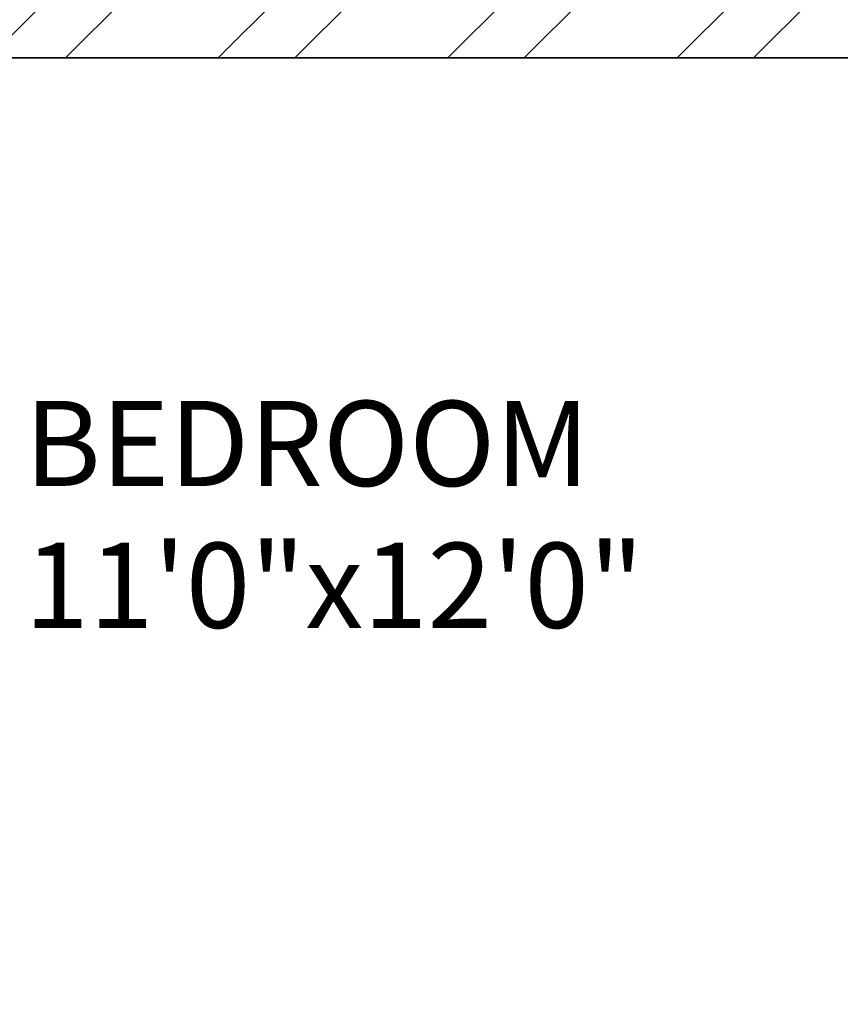
# Model space of a CAD drawing. Units: inches. Extents: x 1962 to 2771, y 1245 to 2660.
# Tile 50 of 114: x 2112 to 2160, y 2122 to 2180. Entities that reach past the tile are written whole.
import ezdxf

# ---------------------------------------------------------------- set-up
doc = ezdxf.new("R2010")
doc.units = ezdxf.units.IN
for name, color, linetype, lineweight in [('A-ANNO-DIMS', 2, 'Continuous', 18), ('A-AREA-IDEN', 7, 'Continuous', 18), ('A-WALL', 7, 'Continuous', 35), ('A-WALL-PATT', 252, 'Continuous', 13)]:
    doc.layers.add(name, color=color, linetype=linetype, lineweight=lineweight)
doc.styles.get("Standard").update_dxf_attribs({"font": 'arial.ttf'})
doc.dimstyles.get("Standard").update_dxf_attribs({"dimtxt": 0.18, "dimasz": 0.18, "dimexe": 0.18, "dimexo": 0.0625, "dimgap": 0.09, "dimtad": 0, "dimtih": 1, "dimtoh": 1, "dimdec": 4, "dimzin": 0, "dimdsep": 46, "dimtxsty": 'Standard', "dimcen": 0.09, "dimadec": 0, "dimazin": 0, "dimtfac": 1, "dimtdec": 4, "dimtofl": 0, "dimtmove": 0, "dimatfit": 3, "dimfxl": 1, "dimtolj": 1, "dimtzin": 0, "dimarcsym": 0})

# ---------------------------------------------------------------- blocks, each defined once
blk = doc.blocks.new('*D40')
at = {"layer": 'A-ANNO-DIMS', "color": 0, "lineweight": -2, "transparency": 16777216}
for p, q in [((2072.02, 2033.906), (2072.02, 2583.474)), ((2072.2, 2583.294), (2366.02, 2583.294)), ((2660.627, 2583.294), (2366.808, 2583.294)), ((2660.807, 2524.406), (2660.807, 2583.474))]:
    blk.add_line(p, q, dxfattribs=at)
at = {"layer": 'A-ANNO-DIMS', "color": 0, "transparency": 16777216}
for points in [[(2072.2, 2583.324), (2072.2, 2583.264), (2072.02, 2583.294)], [(2660.627, 2583.324), (2660.627, 2583.264), (2660.807, 2583.294)]]:
    blk.add_solid(points, dxfattribs=at)
at = {"layer": 'Defpoints', "color": 0, "transparency": 16777216}
for p in [(2660.807, 2583.294), (2660.807, 2524.344), (2072.02, 2033.844)]:
    blk.add_point(p, dxfattribs=at)
at = {"layer": 'A-ANNO-DIMS', "color": 0, "transparency": 16777216, "insert": (2366.414, 2583.294), "char_height": 0.18, "attachment_point": 5}
blk.add_mtext('\\A1;588.8', dxfattribs=at)

msp = doc.modelspace()

# ---------------------------------------------------------------- hatches: boundary and pattern name
at = {"layer": 'A-WALL-PATT'}
h = msp.add_hatch(dxfattribs=at)
h.set_pattern_fill('ANSI32', color=256)
h.paths.add_polyline_path([(2090.8074, 2467.3437), (2141.6481, 2467.3437), (2141.6481, 2469.5937), (2141.6481, 2471.8437), (2086.3074, 2471.8437), (2086.3074, 2422.5333), (2090.8074, 2422.5333)])
h.paths.add_polyline_path([(2282.7664, 2471.8437), (2204.8982, 2471.8437), (2204.8982, 2467.3437), (2234.8074, 2467.3437), (2234.8074, 2311.3437), (2228.7492, 2311.3437), (2228.7492, 2306.8437), (2234.8074, 2306.8437), (2331.9227, 2306.8437), (2331.9227, 2309.0937), (2331.9227, 2311.3437), (2239.3074, 2311.3437), (2239.3074, 2467.3437), (2282.7664, 2467.3437), (2282.7664, 2469.5937)])
h.paths.add_polyline_path([(2471.4531, 2519.8437), (2552.011, 2519.8437), (2564.3996, 2519.8437), (2564.3996, 2511.1389), (2568.8996, 2511.1389), (2568.8996, 2524.3437), (2466.9531, 2524.3437), (2466.9531, 2471.8437), (2450.0749, 2471.8437), (2446.4672, 2471.8437), (2446.4672, 2467.3437), (2450.0749, 2467.3437), (2475.9988, 2467.3437), (2475.9988, 2469.5937), (2475.9988, 2471.8437), (2471.4531, 2471.8437)])
h.paths.add_polyline_path([(2575.2231, 2469.5937), (2575.2231, 2471.8437), (2568.8996, 2471.8437), (2568.8996, 2487.1389), (2564.3996, 2487.1389), (2564.3996, 2471.8437), (2556.511, 2471.8437), (2499.2904, 2471.8437), (2499.2904, 2467.3437), (2507.8074, 2467.3437), (2507.8074, 2311.3437), (2414.863, 2311.3437), (2414.863, 2306.8437), (2512.3074, 2306.8437), (2517.0114, 2306.8437), (2517.0114, 2309.0937), (2517.0114, 2311.3437), (2512.3074, 2311.3437), (2512.3074, 2467.3437), (2575.2231, 2467.3437)])
h.paths.add_polyline_path([(2660.8074, 2471.8437), (2600.9602, 2471.8437), (2600.9602, 2467.3437), (2656.3074, 2467.3437), (2656.3074, 2432.5704), (2660.8074, 2432.5704)])
h.paths.add_polyline_path([(2660.8074, 2372.5704), (2656.3074, 2372.5704), (2656.3074, 2311.3437), (2600.276, 2311.3437), (2600.276, 2309.0937), (2600.276, 2306.8437), (2656.3074, 2306.8437), (2656.3074, 2296.2593), (2660.8074, 2296.2593)])
h.paths.add_polyline_path([(2572.3074, 2306.8437), (2577.1385, 2306.8437), (2577.1385, 2311.3437), (2551.082, 2311.3437), (2551.082, 2306.8437), (2567.8074, 2306.8437), (2567.8074, 2258.8437), (2540.0574, 2258.8437), (2540.0574, 2256.5937), (2540.0574, 2254.3437), (2567.8074, 2254.3437), (2656.3074, 2254.3437), (2656.3074, 2236.9085), (2660.8074, 2236.9085), (2660.8074, 2272.2593), (2656.3074, 2272.2593), (2656.3074, 2258.8437), (2572.3074, 2258.8437)])
h.paths.add_polyline_path([(2512.3074, 2254.3437), (2518.8716, 2254.3437), (2518.8716, 2256.5937), (2518.8716, 2258.8437), (2507.8074, 2258.8437), (2507.8074, 2177.8437), (2567.8074, 2177.8437), (2567.8074, 2172.9628), (2572.3074, 2172.9628), (2572.3074, 2177.8437), (2656.3074, 2177.8437), (2656.3074, 2166.4846), (2660.8074, 2166.4846), (2660.8074, 2200.9085), (2656.3074, 2200.9085), (2656.3074, 2182.3437), (2512.3074, 2182.3437)])
h.paths.add_polyline_path([(2656.3074, 2129.8437), (2572.3074, 2129.8437), (2572.3074, 2150.3044), (2570.0574, 2150.3044), (2567.8074, 2150.3044), (2567.8074, 2129.8437), (2507.8074, 2129.8437), (2507.8074, 2116.3027), (2510.0574, 2116.3027), (2512.3074, 2116.3027), (2512.3074, 2125.3437), (2567.8074, 2125.3437), (2572.3074, 2125.3437), (2656.3074, 2125.3437)])
h.paths.add_polyline_path([(2090.8074, 2362.5333), (2086.3074, 2362.5333), (2086.3074, 2298.6242), (2090.8074, 2298.6242), (2090.8074, 2306.8437), (2174.8074, 2306.8437), (2174.8074, 2286.4178), (2179.3074, 2286.4178), (2179.3074, 2306.8437), (2192.8641, 2306.8437), (2192.8641, 2309.0937), (2192.8641, 2311.3437), (2090.8074, 2311.3437)])
h.paths.add_polyline_path([(2209.156, 2258.8437), (2179.3074, 2258.8437), (2179.3074, 2263.2236), (2177.0574, 2263.2236), (2174.8074, 2263.2236), (2174.8074, 2258.8437), (2090.8074, 2258.8437), (2090.8074, 2274.6242), (2086.3074, 2274.6242), (2086.3074, 2238.2967), (2088.5574, 2238.2967), (2090.8074, 2238.2967), (2090.8074, 2254.3437), (2209.156, 2254.3437)])
h.paths.add_polyline_path([(2090.8074, 2177.8437), (2234.8074, 2177.8437), (2234.8074, 2173.1428), (2239.3074, 2173.1428), (2239.3074, 2258.8437), (2230.8442, 2258.8437), (2230.8442, 2256.5937), (2230.8442, 2254.3437), (2234.8074, 2254.3437), (2234.8074, 2182.3437), (2090.8074, 2182.3437), (2090.8074, 2202.2967), (2086.3074, 2202.2967), (2086.3074, 2140.0389), (2090.8074, 2140.0389)])
h.paths.add_polyline_path([(2090.8074, 2080.0389), (2086.3074, 2080.0389), (2086.3074, 2033.8437), (2090.8074, 2033.8437)], flags=17)
h.paths.add_polyline_path([(2244.9405, 2033.8437), (2239.3074, 2033.8437), (2239.3074, 2142.0665), (2237.2592, 2142.0665), (2234.8074, 2142.0665), (2234.8074, 2033.8437), (2090.8074, 2033.8437), (2076.5204, 2033.8437), (2072.0204, 2033.8437), (2072.0204, 2000.4493), (2076.5204, 2000.4493), (2076.5204, 2029.3437), (2090.8074, 2029.3437), (2244.9405, 2029.3437), (2244.9405, 2031.5937)])
h.paths.add_polyline_path([(2234.8074, 1933.3437), (2076.5204, 1933.3437), (2076.5204, 1952.4493), (2074.2704, 1952.4493), (2072.0204, 1952.4493), (2072.0204, 1933.3437), (2072.0204, 1928.8437), (2234.8074, 1928.8437)])
h.paths.add_polyline_path([(2090.8074, 1928.8437), (2086.3074, 1928.8437), (2086.3074, 1906.5013), (2090.8074, 1906.5013)])
h.paths.add_polyline_path([(2090.8074, 1846.5013), (2086.3074, 1846.5013), (2086.3074, 1769.9917), (2088.5574, 1769.9917), (2090.8074, 1769.9917), (2090.8074, 1780.3437), (2234.8074, 1780.3437), (2234.8074, 1708.3437), (2230.3764, 1708.3437), (2230.3764, 1703.8437), (2239.3074, 1703.8437), (2239.3074, 1792.6669), (2237.0574, 1792.6669), (2234.8074, 1792.6669), (2234.8074, 1784.8437), (2090.8074, 1784.8437)])
h.paths.add_polyline_path([(2239.3074, 1928.8437), (2244.9405, 1928.8437), (2244.9405, 1931.0937), (2244.9405, 1933.3437), (2234.8074, 1933.3437), (2234.8074, 1928.8437), (2234.8074, 1825.5949), (2239.3074, 1825.5949)])
h.paths.add_polyline_path([(2148.0425, 1649.0937), (2148.0425, 1651.3437), (2090.8074, 1651.3437), (2090.8074, 1646.8437), (2148.0425, 1646.8437)], flags=0)
h.paths.add_polyline_path([(2207.5601, 1708.3437), (2090.8074, 1708.3437), (2090.8074, 1703.8437), (2174.8074, 1703.8437), (2174.8074, 1651.3437), (2170.4457, 1651.3437), (2170.4457, 1646.8437), (2195.9924, 1646.8437), (2195.9924, 1649.0937), (2195.9924, 1651.3437), (2179.3074, 1651.3437), (2179.3074, 1703.8437), (2207.5601, 1703.8437), (2207.5601, 1706.0937)])
h.paths.add_polyline_path([(2090.8074, 1733.9917), (2086.3074, 1733.9917), (2086.3074, 1696.1032), (2088.5574, 1696.1032), (2090.8074, 1696.1032)])
h.paths.add_polyline_path([(2090.8074, 1672.1032), (2086.3074, 1672.1032), (2086.3074, 1600.3335), (2090.8074, 1600.3335)])
h.paths.add_polyline_path([(2090.8074, 1540.3335), (2086.3074, 1540.3335), (2086.3074, 1486.3437), (2139.6766, 1486.3437), (2139.6766, 1490.8437), (2090.8074, 1490.8437)])
h.paths.add_polyline_path([(2302.3876, 1490.8437), (2239.3074, 1490.8437), (2239.3074, 1646.8437), (2335.9994, 1646.8437), (2335.9994, 1651.3437), (2229.884, 1651.3437), (2229.884, 1646.8437), (2234.8074, 1646.8437), (2234.8074, 1490.8437), (2202.7103, 1490.8437), (2202.7103, 1488.5937), (2202.7103, 1486.3437), (2275.0699, 1486.3437), (2275.0699, 1475.772), (2279.5699, 1475.772), (2279.5699, 1486.3437), (2302.3876, 1486.3437)])
h.paths.add_polyline_path([(2279.5699, 1451.772), (2275.0699, 1451.772), (2275.0699, 1438.3437), (2174.8074, 1438.3437), (2174.8074, 1486.3437), (2179.7922, 1486.3437), (2179.7922, 1490.8437), (2163.3585, 1490.8437), (2163.3585, 1488.5937), (2163.3585, 1486.3437), (2170.3074, 1486.3437), (2170.3074, 1433.8437), (2279.5699, 1433.8437)])
h.paths.add_polyline_path([(2427.2363, 1490.8437), (2375.8074, 1490.8437), (2375.8074, 1646.8437), (2381.6401, 1646.8437), (2381.6401, 1651.3437), (2365.887, 1651.3437), (2365.887, 1649.0937), (2365.887, 1646.8437), (2371.3074, 1646.8437), (2371.3074, 1490.8437), (2327.5627, 1490.8437), (2327.5627, 1488.5937), (2327.5627, 1486.3437), (2371.3074, 1486.3437), (2371.3074, 1433.8437), (2375.8074, 1433.8437), (2375.8074, 1486.3437), (2427.2363, 1486.3437)])
h.paths.add_polyline_path([(2512.3074, 1646.8437), (2519.4351, 1646.8437), (2519.4351, 1649.0937), (2519.4351, 1651.3437), (2507.8074, 1651.3437), (2416.0063, 1651.3437), (2416.0063, 1649.0937), (2416.0063, 1646.8437), (2507.8074, 1646.8437), (2507.8074, 1490.8437), (2497.0532, 1490.8437), (2497.0532, 1488.5937), (2497.0532, 1486.3437), (2574.9344, 1486.3437), (2574.9344, 1476.0181), (2579.4344, 1476.0181), (2579.4344, 1486.3437), (2584.4872, 1486.3437), (2584.3074, 1490.8437), (2512.3074, 1490.8437)])
h.paths.add_polyline_path([(2470.5091, 1486.3437), (2473.9767, 1486.3437), (2473.9767, 1490.8437), (2449.6605, 1490.8437), (2449.6605, 1488.5937), (2449.6605, 1486.3437), (2466.0091, 1486.3437), (2466.0091, 1433.8437), (2470.5091, 1433.8437), (2579.4344, 1433.8437), (2579.4344, 1452.0181), (2574.9344, 1452.0181), (2574.9344, 1438.3437), (2554.5091, 1438.3437), (2470.5091, 1438.3437)])
h.paths.add_polyline_path([(2656.3074, 1490.8437), (2611.86, 1490.8437), (2611.86, 1486.3437), (2656.3074, 1486.3437)])
h.paths.add_polyline_path([(2660.8074, 1532.7007), (2658.5574, 1532.7007), (2656.3074, 1532.7007), (2656.3074, 1486.3437), (2660.8074, 1486.3437)])
h.paths.add_polyline_path([(2660.8074, 1664.9663), (2656.3074, 1664.9663), (2656.3074, 1651.3437), (2602.2313, 1651.3437), (2602.2313, 1646.8437), (2656.3074, 1646.8437), (2656.3074, 1592.7007), (2660.8074, 1592.7007)])
h.paths.add_polyline_path([(2660.8074, 1724.5221), (2656.3074, 1724.5221), (2656.3074, 1703.8437), (2542.4725, 1703.8437), (2542.4725, 1699.3437), (2567.8074, 1699.3437), (2567.8074, 1651.3437), (2552.7766, 1651.3437), (2552.7766, 1649.0937), (2552.7766, 1646.8437), (2577.2878, 1646.8437), (2577.2878, 1649.0937), (2577.2878, 1651.3437), (2572.3074, 1651.3437), (2572.3074, 1699.3437), (2656.3074, 1699.3437), (2656.3074, 1688.9663), (2660.8074, 1688.9663)])
h.paths.add_polyline_path([(2660.8074, 1880.6524), (2656.3074, 1880.6524), (2656.3074, 1832.8437), (2512.3074, 1832.8437), (2512.3074, 1837.8959), (2507.8074, 1837.8959), (2507.8074, 1828.3437), (2567.8074, 1828.3437), (2567.8074, 1804.3437), (2572.3074, 1804.3437), (2572.3074, 1828.3437), (2656.3074, 1828.3437), (2656.3074, 1818.6778), (2660.8074, 1818.6778)])
h.paths.add_polyline_path([(2660.8074, 1794.6778), (2656.3074, 1794.6778), (2656.3074, 1780.3437), (2572.3074, 1780.3437), (2572.3074, 1783.0303), (2570.0574, 1783.0303), (2567.8074, 1783.0303), (2567.8074, 1780.3437), (2507.8074, 1780.3437), (2507.8074, 1699.3437), (2517.8858, 1699.3437), (2517.8858, 1701.5937), (2517.8858, 1703.8437), (2512.3074, 1703.8437), (2512.3074, 1775.8437), (2656.3074, 1775.8437), (2656.3074, 1760.5221), (2660.8074, 1760.5221)])
h.paths.add_polyline_path([(2660.8074, 1981.3437), (2660.8074, 2020.2808), (2658.5574, 2020.2808), (2656.3074, 2020.2808), (2656.3074, 1981.3437), (2512.3074, 1981.3437), (2512.3074, 2086.6996), (2507.8074, 2086.6996), (2507.8074, 1981.3437), (2375.8074, 1981.3437), (2375.8074, 1986.8505), (2373.5574, 1986.8505), (2371.3074, 1986.8505), (2371.3074, 1973.2607), (2375.8074, 1973.2607), (2375.8074, 1976.8437), (2507.8074, 1976.8437), (2507.8074, 1865.4281), (2510.0574, 1865.4281), (2512.3074, 1865.4281), (2512.3074, 1976.8437), (2660.8074, 1976.8437)])
h.paths.add_polyline_path([(2375.8074, 1940.297), (2373.5574, 1940.297), (2371.3074, 1940.297), (2371.3074, 1933.3437), (2278.4434, 1933.3437), (2278.4434, 1928.8437), (2371.3074, 1928.8437), (2371.3074, 1651.3437), (2375.8074, 1651.3437)])
h.paths.add_polyline_path([(2660.8074, 1976.8437), (2656.3074, 1976.8437), (2656.3074, 1940.6524), (2660.8074, 1940.6524)], flags=17)
h.paths.add_polyline_path([(2660.8074, 2142.4846), (2656.3074, 2142.4846), (2656.3074, 2080.2808), (2660.8074, 2080.2808)])
h.paths.add_polyline_path([(2381.4189, 2311.3437), (2375.8074, 2311.3437), (2375.8074, 2467.3437), (2424.7242, 2467.3437), (2424.7242, 2469.5937), (2424.7242, 2471.8437), (2375.8074, 2471.8437), (2375.8074, 2524.3437), (2371.3074, 2524.3437), (2371.3074, 2471.8437), (2307.2097, 2471.8437), (2307.2097, 2467.3437), (2371.3074, 2467.3437), (2371.3074, 2311.3437), (2366.8901, 2311.3437), (2366.8901, 2306.8437), (2371.3074, 2306.8437), (2371.3074, 2033.8437), (2279.6589, 2033.8437), (2279.6589, 2029.3437), (2371.3074, 2029.3437), (2371.3074, 2014.2598), (2375.8074, 2014.2598), (2375.8074, 2306.8437), (2381.4189, 2306.8437)])
h.paths.add_polyline_path([(2263.3074, 2524.3437), (2170.3074, 2524.3437), (2170.3074, 2519.8437), (2170.3074, 2471.8437), (2165.0312, 2471.8437), (2165.0312, 2467.3437), (2179.6721, 2467.3437), (2179.6721, 2469.5161), (2179.6721, 2471.8437), (2174.8074, 2471.8437), (2174.8074, 2519.8437), (2258.8074, 2519.8437), (2258.8074, 2511.6436), (2263.3074, 2511.6436)])
h.paths.add_polyline_path([(2245.0232, 1361.4123), (2492.9468, 1361.4123), (2492.9468, 1398.505), (2245.0232, 1398.505)], flags=9)
h.paths.add_polyline_path([(2388.1434, 2086.6936), (2425.0704, 2086.6936), (2425.0704, 2105.3509), (2388.1434, 2105.3509)], flags=9)
h.paths.add_polyline_path([(2404.922, 2242.6744), (2445.7337, 2242.6744), (2445.7337, 2261.3318), (2404.922, 2261.3318)], flags=9)
h.paths.add_polyline_path([(2269.4107, 2156.7935), (2306.3378, 2156.7935), (2306.3378, 2175.4508), (2269.4107, 2175.4508)], flags=9)
h.paths.add_polyline_path([(2269.3277, 2233.4343), (2306.2547, 2233.4343), (2306.2547, 2252.0917), (2269.3277, 2252.0917)], flags=9)
h.paths.add_polyline_path([(2431.6052, 2320.6922), (2470.4456, 2320.6922), (2470.4456, 2339.3495), (2431.6052, 2339.3495)], flags=25)
h.paths.add_polyline_path([(2249.6902, 2315.7608), (2288.5306, 2315.7608), (2288.5306, 2334.4182), (2249.6902, 2334.4182)], flags=25)
h.paths.add_polyline_path([(2096.9301, 2314.3181), (2135.7704, 2314.3181), (2135.7704, 2332.9755), (2096.9301, 2332.9755)], flags=25)
h.paths.add_polyline_path([(2134.3475, 2285.7089), (2161.4655, 2285.7089), (2161.4655, 2304.3662), (2134.3475, 2304.3662)], flags=9)
h.paths.add_polyline_path([(2126.5155, 2209.4076), (2159.9227, 2209.4076), (2159.9227, 2228.065), (2126.5155, 2228.065)], flags=25)
h.paths.add_polyline_path([(2110.5753, 2141.5299), (2149.4157, 2141.5299), (2149.4157, 2160.1872), (2110.5753, 2160.1872)], flags=25)
h.paths.add_polyline_path([(2249.8618, 1968.3317), (2286.3966, 1968.3317), (2286.3966, 1986.989), (2249.8618, 1986.989)], flags=9)
h.paths.add_polyline_path([(2395.9507, 1777.0051), (2436.7624, 1777.0051), (2436.7624, 1795.6625), (2395.9507, 1795.6625)], flags=9)
h.paths.add_polyline_path([(2398.5259, 1888.5651), (2435.0062, 1888.5651), (2435.0062, 1907.2224), (2398.5259, 1907.2224)], flags=25)
h.paths.add_polyline_path([(2259.3506, 1728.3559), (2296.2776, 1728.3559), (2296.2776, 1747.0132), (2259.3506, 1747.0132)], flags=9)
h.paths.add_polyline_path([(2271.3698, 1845.268), (2308.2968, 1845.268), (2308.2968, 1863.9253), (2271.3698, 1863.9253)], flags=9)
h.paths.add_polyline_path([(2120.9355, 1786.3027), (2159.7759, 1786.3027), (2159.7759, 1804.9601), (2120.9355, 1804.9601)], flags=25)
h.paths.add_polyline_path([(2121.3164, 1732.1043), (2154.7236, 1732.1043), (2154.7236, 1750.7616), (2121.3164, 1750.7616)], flags=25)
h.paths.add_polyline_path([(2118.3706, 1678.8997), (2147.5282, 1678.8997), (2147.5282, 1697.557), (2118.3706, 1697.557)], flags=25)
h.paths.add_polyline_path([(2385.9227, 1493.557), (2424.763, 1493.557), (2424.763, 1512.2143), (2385.9227, 1512.2143)], flags=25)
h.paths.add_polyline_path([(2248.7058, 1500.0256), (2287.5462, 1500.0256), (2287.5462, 1518.6829), (2248.7058, 1518.6829)], flags=25)
h.paths.add_polyline_path([(2104.1669, 1617.3771), (2143.0073, 1617.3771), (2143.0073, 1636.0344), (2104.1669, 1636.0344)], flags=9)
h.paths.add_polyline_path([(2096.0714, 1447.8824), (2137.3845, 1447.8824), (2137.3845, 1458.1859), (2096.0714, 1458.1859)], flags=9)
h.paths.add_polyline_path([(2180.6114, 1440.325), (2209.7689, 1440.325), (2209.7689, 1458.9823), (2180.6114, 1458.9823)], flags=25)
h.paths.add_polyline_path([(2316.1698, 1447.9637), (2357.4829, 1447.9637), (2357.4829, 1458.2673), (2316.1698, 1458.2673)], flags=9)
h.paths.add_polyline_path([(2397.6187, 1447.9637), (2438.9318, 1447.9637), (2438.9318, 1458.2673), (2397.6187, 1458.2673)], flags=9)
h.paths.add_polyline_path([(2473.0778, 1439.5953), (2502.2354, 1439.5953), (2502.2354, 1458.2527), (2473.0778, 1458.2527)], flags=25)
h.paths.add_polyline_path([(2589.7027, 1447.8819), (2631.0158, 1447.8819), (2631.0158, 1458.1855), (2589.7027, 1458.1855)], flags=9)
h.paths.add_polyline_path([(2522.4009, 1497.5285), (2561.2413, 1497.5285), (2561.2413, 1516.1859), (2522.4009, 1516.1859)], flags=25)
h.paths.add_polyline_path([(2579.6565, 1671.3482), (2608.8141, 1671.3482), (2608.8141, 1690.0056), (2579.6565, 1690.0056)], flags=25)
h.paths.add_polyline_path([(2544.7038, 1725.5064), (2578.1111, 1725.5064), (2578.1111, 1744.1637), (2544.7038, 1744.1637)], flags=25)
h.paths.add_polyline_path([(2578.1191, 1807.472), (2607.2766, 1807.472), (2607.2766, 1826.1293), (2578.1191, 1826.1293)], flags=25)
h.paths.add_polyline_path([(2595.0614, 1835.1839), (2633.9018, 1835.1839), (2633.9018, 1853.8413), (2595.0614, 1853.8413)], flags=25)
h.paths.add_polyline_path([(2567.0097, 2097.7035), (2605.8501, 2097.7035), (2605.8501, 2116.3609), (2567.0097, 2116.3609)], flags=9)
h.paths.add_polyline_path([(2586.644, 2134.6454), (2615.8015, 2134.6454), (2615.8015, 2153.3027), (2586.644, 2153.3027)], flags=9)
h.paths.add_polyline_path([(2544.6185, 2212.6783), (2578.0258, 2212.6783), (2578.0258, 2231.3356), (2544.6185, 2231.3356)], flags=25)
h.paths.add_polyline_path([(2577.0273, 2256.9023), (2606.1849, 2256.9023), (2606.1849, 2275.5597), (2577.0273, 2275.5597)], flags=24)
h.paths.add_polyline_path([(2605.2683, 2315.2821), (2644.1087, 2315.2821), (2644.1087, 2333.9395), (2605.2683, 2333.9395)], flags=25)
h.paths.add_polyline_path([(2583.1244, 2496.1815), (2624.4375, 2496.1815), (2624.4375, 2506.4851), (2583.1244, 2506.4851)], flags=9)
h.paths.add_polyline_path([(2474.761, 2497.0823), (2503.9185, 2497.0823), (2503.9185, 2515.7397), (2474.761, 2515.7397)], flags=25)
h.paths.add_polyline_path([(2387.5787, 2494.2563), (2428.902, 2494.2563), (2428.902, 2504.5598), (2387.5787, 2504.5598)], flags=9)
h.paths.add_polyline_path([(2300.1657, 2500.1564), (2341.4788, 2500.1564), (2341.4788, 2510.46), (2300.1657, 2510.46)], flags=25)
h.paths.add_polyline_path([(2176.8589, 2497.5843), (2206.0165, 2497.5843), (2206.0165, 2516.2416), (2176.8589, 2516.2416)], flags=25)
h.paths.add_polyline_path([(2097.4668, 2494.9762), (2138.7799, 2494.9762), (2138.7799, 2505.2798), (2097.4668, 2505.2798)], flags=9)

# ---------------------------------------------------------------- linework, layer by layer
at = {"layer": 'A-WALL'}
msp.add_line((2090.8074, 2177.8437), (2234.8074, 2177.8437), dxfattribs=at)

# ---------------------------------------------------------------- texts
at = {"layer": 'A-AREA-IDEN', "insert": (2112.5859, 2157.7026), "char_height": 5, "attachment_point": 1}
msp.add_mtext_dynamic_manual_height_columns('BEDROOM\\P11\'0"x12\'0"', width=221.156008, gutter_width=12.5, heights=[0], dxfattribs=at)

# ---------------------------------------------------------------- dimensions: what is measured, and where the dimension line sits
at = {"layer": 'A-ANNO-DIMS'}
dim = msp.add_linear_dim(base=(2660.8074, 2583.2937), p1=(2072.0204, 2033.8437), p2=(2660.8074, 2524.3437), dimstyle='Standard', override={"dimdec": 1, "dimlfac": 1, "dimrnd": 0, "dimzin": 0, "dimdsep": 46, "dimlunit": 2}, dxfattribs=at)
dim.commit()
dim.dimension.update_dxf_attribs({"geometry": '*D40', "text_midpoint": (2366.4139, 2583.2937)})

doc.saveas('drawing.dxf')
